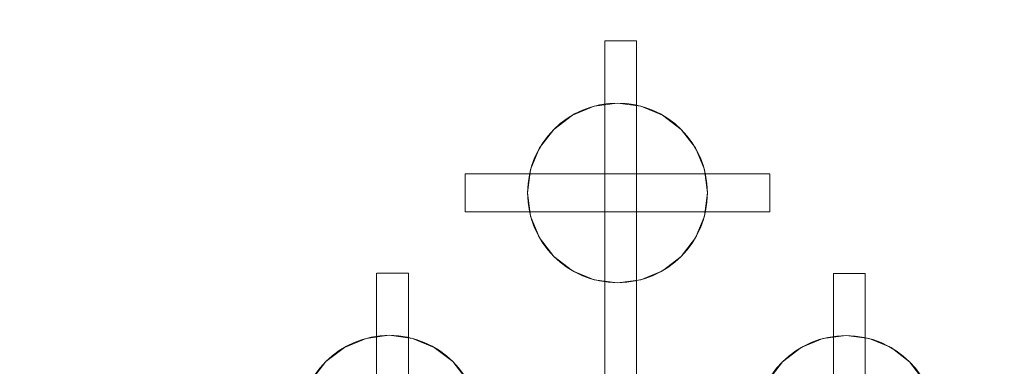
# Model space of a CAD drawing. Units: inches. Extents: x 2696 to 3240, y 1564 to 2310.
# Tile 57 of 76: x 2907.148 to 2916.848, y 2188.894 to 2192.312. Entities that reach past the tile are written whole.
import ezdxf

# ---------------------------------------------------------------- set-up
doc = ezdxf.new("R2010")
doc.units = ezdxf.units.IN
for name, color, linetype, lineweight in [('A-ANNO-DIMS', 3, 'Continuous', 18), ('A-FLOR-FIXT', 8, 'Continuous', 18), ('A-FURN', 251, 'Continuous', 13)]:
    doc.layers.add(name, color=color, linetype=linetype, lineweight=lineweight)
doc.layers.add('FURNITURE', color=250, linetype='Continuous')
doc.styles.add('TIMES NEW', font='times.ttf')
doc.dimstyles.new('Siddhuu', dxfattribs={"dimtxt": 6, "dimasz": 2.5, "dimexe": 1.25, "dimexo": 0.625, "dimtad": 1, "dimdec": 1, "dimlunit": 4, "dimtxsty": 'TIMES NEW', "dimcen": 2.5, "dimclrd": 256, "dimclre": 1, "dimclrt": 7, "dimadec": 0, "dimazin": 0, "dimtfac": 1, "dimtdec": 1, "dimtmove": 0, "dimatfit": 3, "dimfxl": 1, "dimtolj": 1, "dimlwd": -1, "dimarcsym": 0})

# ---------------------------------------------------------------- blocks, each defined once
blk = doc.blocks.new('A$C1af1f523')
at = {"layer": 'A-FURN'}
for p, q in [((-2.9003, 3.9351), (-2.9003, 0.9365)), ((-2.9003, 3.9351, 0.5), (-2.9003, 0.9365, 0.5)), ((-2.9003, 3.9351), (-2.9003, 3.9351, 0.5)), ((-2.5253, 3.9351), (-2.9003, 3.9351)), ((-2.5253, 3.9351, 0.5), (-2.9003, 3.9351, 0.5)), ((-2.5253, 3.9351), (-2.5253, 0.9365)), ((-2.5253, 3.9351, 0.5), (-2.5253, 0.9365, 0.5)), ((-2.5253, 3.9351), (-2.5253, 3.9351, 0.5)), ((-2.7128, 3.3215), (-2.7128, 3.3215, 0.5)), ((-3.1558, 3.2028), (-3.1558, 3.2028, 0.5)), ((-2.9421, 3.2913), (-2.9421, 3.2913, 0.5)), ((-2.4835, 3.2913), (-2.4835, 3.2913, 0.5)), ((-2.2698, 3.2028), (-2.2698, 3.2028, 0.5)), ((-3.3393, 3.062), (-3.3393, 3.062, 0.5)), ((-2.0863, 3.062), (-2.0863, 3.062, 0.5)), ((-3.4801, 2.8785), (-3.4801, 2.8785, 0.5)), ((-1.9455, 2.8785), (-1.9455, 2.8785, 0.5)), ((-3.5686, 2.6648), (-3.5686, 2.6648, 0.5)), ((-1.857, 2.6648), (-1.857, 2.6648, 0.5)), ((0, 2.5605), (-4.2116, 2.5605)), ((0, 2.5605, 0.5), (-4.2116, 2.5605, 0.5)), ((-4.2116, 2.5605), (-4.2116, 2.5605, 0.5)), ((-4.2116, 2.5594), (-4.2116, 2.248)), ((-4.2116, 2.5594, 0.5), (-4.2116, 2.248, 0.5)), ((-4.2116, 2.5594), (-4.2116, 2.5594, 0.5)), ((-3.5988, 2.4355), (-3.5988, 2.4355, 0.5)), ((-1.8268, 2.4355), (-1.8268, 2.4355, 0.5)), ((0, 2.248), (-4.2116, 2.248)), ((0, 2.248, 0.5), (-4.2116, 2.248, 0.5)), ((-4.2116, 2.248), (-4.2116, 2.248, 0.5)), ((-4.2116, 2.248), (-4.2116, 2.2469)), ((-4.2116, 2.248, 0.5), (-4.2116, 2.2469, 0.5)), ((-4.2116, 2.2469), (-4.2116, 2.2469, 0.5)), ((-3.5686, 2.2061), (-3.5686, 2.2061, 0.5)), ((-1.857, 2.2061), (-1.857, 2.2061, 0.5)), ((-3.4801, 1.9924), (-3.4801, 1.9924, 0.5)), ((-1.9455, 1.9924), (-1.9455, 1.9924, 0.5)), ((-3.3393, 1.8089), (-3.3393, 1.8089, 0.5)), ((-2.0863, 1.8089), (-2.0863, 1.8089, 0.5)), ((-4.8156, 1.6871), (-5.1906, 1.6871)), ((-4.8156, 1.6871, 0.5), (-5.1906, 1.6871, 0.5)), ((-5.1906, 1.6871), (-5.1906, 1.6871, 0.5)), ((-5.1906, 1.6871), (-5.1901, -1.3115)), ((-5.1906, 1.6871, 0.5), (-5.1901, -1.3115, 0.5)), ((-4.8156, 1.6871), (-4.8156, 1.6871, 0.5)), ((-4.8156, 1.6871), (-4.8151, -1.3115)), ((-4.8156, 1.6871, 0.5), (-4.8151, -1.3115, 0.5)), ((-3.1558, 1.6681), (-3.1558, 1.6681, 0.5)), ((-2.2698, 1.6681), (-2.2698, 1.6681, 0.5)), ((-2.9421, 1.5796), (-2.9421, 1.5796, 0.5)), ((-2.4835, 1.5796), (-2.4835, 1.5796, 0.5)), ((-2.7128, 1.5494), (-2.7128, 1.5494, 0.5)), ((-5.0026, 1.0735), (-5.0026, 1.0735, 0.5)), ((-5.232, 1.0433), (-5.232, 1.0433, 0.5)), ((-4.7733, 1.0433), (-4.7733, 1.0433, 0.5)), ((-5.4457, 0.9548), (-5.4457, 0.9548, 0.5)), ((-4.5596, 0.9548), (-4.5596, 0.9548, 0.5)), ((-2.9003, 0.9365), (-2.9003, 0.9365, 0.5)), ((-2.5253, 0.9365), (-2.8979, 0.9365)), ((-2.5253, 0.9365, 0.5), (-2.8979, 0.9365, 0.5)), ((-2.8979, 0.9365), (-2.8979, 0.9365, 0.5)), ((-2.5253, 0.9365), (-2.5253, 0.9365, 0.5)), ((-5.6292, 0.814), (-5.6292, 0.814, 0.5)), ((-4.3761, 0.814), (-4.3761, 0.814, 0.5)), ((-5.77, 0.6305), (-5.77, 0.6305, 0.5)), ((-4.2353, 0.6305), (-4.2353, 0.6305, 0.5)), ((-5.8585, 0.4168), (-5.8585, 0.4168, 0.5)), ((-4.1468, 0.4168), (-4.1468, 0.4168, 0.5)), ((0, 0.3125), (-6.5015, 0.3125)), ((0, 0.3125, 0.5), (-6.5015, 0.3125, 0.5)), ((-6.5015, 0.3125), (-6.5015, 0.3125, 0.5)), ((-6.5015, 0.3114), (-6.5015, 0)), ((-6.5015, 0.3114, 0.5), (-6.5015, 0, 0.5)), ((-6.5015, 0.3114), (-6.5015, 0.3114, 0.5)), ((-5.8887, 0.1875), (-5.8887, 0.1875, 0.5)), ((-4.1166, 0.1875), (-4.1166, 0.1875, 0.5)), ((0, 0), (-6.5015, 0)), ((0, 0, 0.5), (-6.5015, 0, 0.5)), ((-6.5015, 0), (-6.5015, 0, 0.5)), ((-6.5015, 0), (-6.5015, -0.0011)), ((-6.5015, 0, 0.5), (-6.5015, -0.0011, 0.5)), ((-6.5015, -0.0011), (-6.5015, -0.0011, 0.5)), ((-5.8585, -0.0418), (-5.8585, -0.0418, 0.5)), ((-4.1468, -0.0418), (-4.1468, -0.0418, 0.5)), ((-5.77, -0.2555), (-5.77, -0.2555, 0.5)), ((-4.2353, -0.2555), (-4.2353, -0.2555, 0.5)), ((-5.6292, -0.439), (-5.6292, -0.439, 0.5)), ((-4.3761, -0.439), (-4.3761, -0.439, 0.5)), ((-5.4457, -0.5798), (-5.4457, -0.5798, 0.5)), ((-4.5596, -0.5798), (-4.5596, -0.5798, 0.5)), ((-2.898, -0.5642), (-2.898, -3.5628)), ((-2.898, -0.5642, 0.5), (-2.898, -3.5628, 0.5)), ((-2.898, -0.5642), (-2.898, -0.5642, 0.5)), ((-2.523, -0.5642), (-2.898, -0.5642)), ((-2.523, -0.5642, 0.5), (-2.898, -0.5642, 0.5)), ((-2.523, -0.5642), (-2.523, -3.5628)), ((-2.523, -0.5642, 0.5), (-2.523, -3.5628, 0.5)), ((-2.523, -0.5642), (-2.523, -0.5642, 0.5)), ((-5.232, -0.6683), (-5.232, -0.6683, 0.5)), ((-4.7733, -0.6683), (-4.7733, -0.6683, 0.5)), ((-5.0026, -0.6985), (-5.0026, -0.6985, 0.5)), ((-2.9398, -1.208), (-2.9398, -1.208, 0.5)), ((-2.7105, -1.1778), (-2.7105, -1.1778, 0.5)), ((-2.4812, -1.208), (-2.4812, -1.208, 0.5)), ((-5.1901, -1.3115), (-5.1901, -1.3115, 0.5)), ((-4.8151, -1.3115), (-5.1878, -1.3115)), ((-4.8151, -1.3115, 0.5), (-5.1878, -1.3115, 0.5)), ((-5.1878, -1.3115), (-5.1878, -1.3115, 0.5)), ((-4.8151, -1.3115), (-4.8151, -1.3115, 0.5)), ((-3.1535, -1.2965), (-3.1535, -1.2965, 0.5)), ((-2.2675, -1.2965), (-2.2675, -1.2965, 0.5)), ((-3.337, -1.4373), (-3.337, -1.4373, 0.5)), ((-2.084, -1.4373), (-2.084, -1.4373, 0.5)), ((-3.4778, -1.6208), (-3.4778, -1.6208, 0.5)), ((-1.9432, -1.6208), (-1.9432, -1.6208, 0.5)), ((-3.5664, -1.8345), (-3.5664, -1.8345, 0.5)), ((-1.8547, -1.8345), (-1.8547, -1.8345, 0.5)), ((0, -1.9388), (-4.2094, -1.9388)), ((0, -1.9388, 0.5), (-4.2094, -1.9388, 0.5)), ((-4.2094, -1.9388), (-4.2094, -1.9388, 0.5)), ((-4.2094, -1.9399), (-4.2094, -2.2513)), ((-4.2094, -1.9399, 0.5), (-4.2094, -2.2513, 0.5)), ((-4.2094, -1.9399), (-4.2094, -1.9399, 0.5)), ((-3.5965, -2.0638), (-3.5965, -2.0638, 0.5)), ((-1.8245, -2.0638), (-1.8245, -2.0638, 0.5)), ((0, -2.2513), (-4.2094, -2.2513)), ((0, -2.2513, 0.5), (-4.2094, -2.2513, 0.5)), ((-4.2094, -2.2513), (-4.2094, -2.2513, 0.5)), ((-4.2094, -2.2513), (-4.2094, -2.2524)), ((-4.2094, -2.2513, 0.5), (-4.2094, -2.2524, 0.5)), ((-4.2094, -2.2524), (-4.2094, -2.2524, 0.5)), ((-3.5664, -2.2931), (-3.5664, -2.2931, 0.5)), ((-1.8547, -2.2931), (-1.8547, -2.2931, 0.5)), ((-3.4778, -2.5068), (-3.4778, -2.5068, 0.5)), ((-1.9432, -2.5068), (-1.9432, -2.5068, 0.5)), ((-3.337, -2.6903), (-3.337, -2.6903, 0.5)), ((-2.084, -2.6903), (-2.084, -2.6903, 0.5)), ((-3.1535, -2.8311), (-3.1535, -2.8311, 0.5)), ((-2.2675, -2.8311), (-2.2675, -2.8311, 0.5)), ((-2.9398, -2.9196), (-2.9398, -2.9196, 0.5)), ((-2.7105, -2.9498), (-2.7105, -2.9498, 0.5)), ((-2.4812, -2.9196), (-2.4812, -2.9196, 0.5)), ((-2.898, -3.5628), (-2.898, -3.5628, 0.5)), ((-2.523, -3.5628), (-2.8956, -3.5628)), ((-2.523, -3.5628, 0.5), (-2.8956, -3.5628, 0.5)), ((-2.8956, -3.5628), (-2.8956, -3.5628, 0.5)), ((-2.523, -3.5628), (-2.523, -3.5628, 0.5))]:
    blk.add_line(p, q, dxfattribs=at)
for centre in [(-2.7128, 2.4355), (-2.7128, 2.4355, 0.5), (-5.0026, 0.1875), (-5.0026, 0.1875, 0.5), (-2.7105, -2.0638), (-2.7105, -2.0638, 0.5)]:
    blk.add_circle(centre, 0.886, dxfattribs=at)
at = {"layer": 'FURNITURE'}
for p, q in [((0, 2.5605), (0, 2.5605, 0.5)), ((0, 2.248), (0, 2.248, 0.5)), ((0, 0.3125), (0, 0.3125, 0.5)), ((0, 0), (0, 0, 0.5)), ((0, -1.9388), (0, -1.9388, 0.5)), ((0, -2.2513), (0, -2.2513, 0.5))]:
    blk.add_line(p, q, dxfattribs=at)
at = {"layer": 'A-FURN'}
mesh = blk.add_polyface(dxfattribs=at)
corners = [(-2.9003, 0.9365, 0.5), (-2.9003, 3.9351), (-2.9003, 0.9365), (-2.9003, 3.9351, 0.5)]
mesh.append_faces([[corners[k] for k in face] for face in [(2, 1, 0), (3, 0, 1)]], dxfattribs={"vtx1": -1})
mesh = blk.add_polyface(dxfattribs=at)
corners = [(-2.5253, 3.9351, 0.5), (-2.9003, 3.9351), (-2.9003, 3.9351, 0.5), (-2.5253, 3.9351)]
mesh.append_faces([[corners[k] for k in face] for face in [(2, 1, 0), (3, 0, 1)]], dxfattribs={"vtx1": -1})
mesh = blk.add_polyface(dxfattribs=at)
corners = [(-2.5253, 0.9365, 0.5), (-2.5253, 3.9351), (-2.5253, 0.9365), (-2.5253, 3.9351, 0.5)]
mesh.append_faces([[corners[k] for k in face] for face in [(2, 1, 0), (3, 0, 1)]], dxfattribs={"vtx1": -1})
mesh = blk.add_polyface(dxfattribs=at)
corners = [(-2.7128, 3.3215), (-2.9421, 3.2913, 0.5), (-2.9421, 3.2913), (-2.7128, 3.3215, 0.5)]
mesh.append_faces([[corners[k] for k in face] for face in [(2, 1, 0), (3, 0, 1)]], dxfattribs={"vtx1": -1})
mesh = blk.add_polyface(dxfattribs=at)
corners = [(-2.4835, 3.2913), (-2.7128, 3.3215, 0.5), (-2.7128, 3.3215), (-2.4835, 3.2913, 0.5)]
mesh.append_faces([[corners[k] for k in face] for face in [(2, 1, 0), (3, 0, 1)]], dxfattribs={"vtx1": -1})
mesh = blk.add_polyface(dxfattribs=at)
corners = [(-3.1558, 3.2028), (-3.3393, 3.062, 0.5), (-3.3393, 3.062), (-3.1558, 3.2028, 0.5)]
mesh.append_faces([[corners[k] for k in face] for face in [(2, 1, 0), (3, 0, 1)]], dxfattribs={"vtx1": -1})
mesh = blk.add_polyface(dxfattribs=at)
corners = [(-2.9421, 3.2913), (-3.1558, 3.2028, 0.5), (-3.1558, 3.2028), (-2.9421, 3.2913, 0.5)]
mesh.append_faces([[corners[k] for k in face] for face in [(2, 1, 0), (3, 0, 1)]], dxfattribs={"vtx1": -1})
mesh = blk.add_polyface(dxfattribs=at)
corners = [(-2.2698, 3.2028), (-2.4835, 3.2913, 0.5), (-2.4835, 3.2913), (-2.2698, 3.2028, 0.5)]
mesh.append_faces([[corners[k] for k in face] for face in [(2, 1, 0), (3, 0, 1)]], dxfattribs={"vtx1": -1})
mesh = blk.add_polyface(dxfattribs=at)
corners = [(-2.0863, 3.062), (-2.2698, 3.2028, 0.5), (-2.2698, 3.2028), (-2.0863, 3.062, 0.5)]
mesh.append_faces([[corners[k] for k in face] for face in [(2, 1, 0), (3, 0, 1)]], dxfattribs={"vtx1": -1})
mesh = blk.add_polyface(dxfattribs=at)
corners = [(-3.3393, 3.062, 0.5), (-3.4801, 2.8785), (-3.3393, 3.062), (-3.4801, 2.8785, 0.5)]
mesh.append_faces([[corners[k] for k in face] for face in [(2, 1, 0), (3, 0, 1)]], dxfattribs={"vtx1": -1})
mesh = blk.add_polyface(dxfattribs=at)
corners = [(-1.9455, 2.8785, 0.5), (-2.0863, 3.062), (-1.9455, 2.8785), (-2.0863, 3.062, 0.5)]
mesh.append_faces([[corners[k] for k in face] for face in [(2, 1, 0), (3, 0, 1)]], dxfattribs={"vtx1": -1})
mesh = blk.add_polyface(dxfattribs=at)
corners = [(-3.4801, 2.8785, 0.5), (-3.5686, 2.6648), (-3.4801, 2.8785), (-3.5686, 2.6648, 0.5)]
mesh.append_faces([[corners[k] for k in face] for face in [(2, 1, 0), (3, 0, 1)]], dxfattribs={"vtx1": -1})
mesh = blk.add_polyface(dxfattribs=at)
corners = [(-1.857, 2.6648, 0.5), (-1.9455, 2.8785), (-1.857, 2.6648), (-1.9455, 2.8785, 0.5)]
mesh.append_faces([[corners[k] for k in face] for face in [(2, 1, 0), (3, 0, 1)]], dxfattribs={"vtx1": -1})
mesh = blk.add_polyface(dxfattribs=at)
corners = [(-3.5686, 2.6648, 0.5), (-3.5988, 2.4355), (-3.5686, 2.6648), (-3.5988, 2.4355, 0.5)]
mesh.append_faces([[corners[k] for k in face] for face in [(2, 1, 0), (3, 0, 1)]], dxfattribs={"vtx1": -1})
mesh = blk.add_polyface(dxfattribs=at)
corners = [(-1.8268, 2.4355, 0.5), (-1.857, 2.6648), (-1.8268, 2.4355), (-1.857, 2.6648, 0.5)]
mesh.append_faces([[corners[k] for k in face] for face in [(2, 1, 0), (3, 0, 1)]], dxfattribs={"vtx1": -1})
mesh = blk.add_polyface(dxfattribs=at)
corners = [(0, 2.5605, 0.5), (-4.2116, 2.5605), (-4.2116, 2.5605, 0.5), (0, 2.5605)]
mesh.append_faces([[corners[k] for k in face] for face in [(2, 1, 0), (3, 0, 1)]], dxfattribs={"vtx1": -1})
mesh = blk.add_polyface(dxfattribs=at)
corners = [(-4.2116, 2.2469, 0.5), (-4.2116, 2.248), (-4.2116, 2.2469), (-4.2116, 2.5594), (-4.2116, 2.5594, 0.5), (-4.2116, 2.248, 0.5)]
mesh.append_faces([[corners[k] for k in face] for face in [(3, 0, 1), (4, 0, 3)]], dxfattribs={"vtx0": -1, "vtx1": -1})
mesh.append_faces([[corners[k] for k in face] for face in [(2, 1, 0), (5, 0, 4)]], dxfattribs={"vtx1": -1})
mesh = blk.add_polyface(dxfattribs=at)
corners = [(-3.5988, 2.4355, 0.5), (-3.5686, 2.2061), (-3.5988, 2.4355), (-3.5686, 2.2061, 0.5)]
mesh.append_faces([[corners[k] for k in face] for face in [(2, 1, 0), (3, 0, 1)]], dxfattribs={"vtx1": -1})
mesh = blk.add_polyface(dxfattribs=at)
corners = [(-1.857, 2.2061, 0.5), (-1.8268, 2.4355), (-1.857, 2.2061), (-1.8268, 2.4355, 0.5)]
mesh.append_faces([[corners[k] for k in face] for face in [(2, 1, 0), (3, 0, 1)]], dxfattribs={"vtx1": -1})
mesh = blk.add_polyface(dxfattribs=at)
corners = [(0, 2.248, 0.5), (-4.2116, 2.248), (-4.2116, 2.248, 0.5), (0, 2.248)]
mesh.append_faces([[corners[k] for k in face] for face in [(2, 1, 0), (3, 0, 1)]], dxfattribs={"vtx1": -1})
mesh = blk.add_polyface(dxfattribs=at)
corners = [(-3.5686, 2.2061, 0.5), (-3.4801, 1.9924), (-3.5686, 2.2061), (-3.4801, 1.9924, 0.5)]
mesh.append_faces([[corners[k] for k in face] for face in [(2, 1, 0), (3, 0, 1)]], dxfattribs={"vtx1": -1})
mesh = blk.add_polyface(dxfattribs=at)
corners = [(-1.9455, 1.9924, 0.5), (-1.857, 2.2061), (-1.9455, 1.9924), (-1.857, 2.2061, 0.5)]
mesh.append_faces([[corners[k] for k in face] for face in [(2, 1, 0), (3, 0, 1)]], dxfattribs={"vtx1": -1})
mesh = blk.add_polyface(dxfattribs=at)
corners = [(-3.4801, 1.9924, 0.5), (-3.3393, 1.8089), (-3.4801, 1.9924), (-3.3393, 1.8089, 0.5)]
mesh.append_faces([[corners[k] for k in face] for face in [(2, 1, 0), (3, 0, 1)]], dxfattribs={"vtx1": -1})
mesh = blk.add_polyface(dxfattribs=at)
corners = [(-2.0863, 1.8089, 0.5), (-1.9455, 1.9924), (-2.0863, 1.8089), (-1.9455, 1.9924, 0.5)]
mesh.append_faces([[corners[k] for k in face] for face in [(2, 1, 0), (3, 0, 1)]], dxfattribs={"vtx1": -1})
mesh = blk.add_polyface(dxfattribs=at)
corners = [(-3.1558, 1.6681, 0.5), (-3.3393, 1.8089), (-3.3393, 1.8089, 0.5), (-3.1558, 1.6681)]
mesh.append_faces([[corners[k] for k in face] for face in [(2, 1, 0), (3, 0, 1)]], dxfattribs={"vtx1": -1})
mesh = blk.add_polyface(dxfattribs=at)
corners = [(-2.0863, 1.8089, 0.5), (-2.2698, 1.6681), (-2.2698, 1.6681, 0.5), (-2.0863, 1.8089)]
mesh.append_faces([[corners[k] for k in face] for face in [(2, 1, 0), (3, 0, 1)]], dxfattribs={"vtx1": -1})
mesh = blk.add_polyface(dxfattribs=at)
corners = [(-4.8156, 1.6871, 0.5), (-5.1906, 1.6871), (-5.1906, 1.6871, 0.5), (-4.8156, 1.6871)]
mesh.append_faces([[corners[k] for k in face] for face in [(2, 1, 0), (3, 0, 1)]], dxfattribs={"vtx1": -1})
mesh = blk.add_polyface(dxfattribs=at)
corners = [(-5.1901, -1.3115, 0.5), (-5.1906, 1.6871), (-5.1901, -1.3115), (-5.1906, 1.6871, 0.5)]
mesh.append_faces([[corners[k] for k in face] for face in [(2, 1, 0), (3, 0, 1)]], dxfattribs={"vtx1": -1})
mesh = blk.add_polyface(dxfattribs=at)
corners = [(-4.8151, -1.3115, 0.5), (-4.8156, 1.6871), (-4.8151, -1.3115), (-4.8156, 1.6871, 0.5)]
mesh.append_faces([[corners[k] for k in face] for face in [(2, 1, 0), (3, 0, 1)]], dxfattribs={"vtx1": -1})
mesh = blk.add_polyface(dxfattribs=at)
corners = [(-2.9421, 1.5796, 0.5), (-3.1558, 1.6681), (-3.1558, 1.6681, 0.5), (-2.9421, 1.5796)]
mesh.append_faces([[corners[k] for k in face] for face in [(2, 1, 0), (3, 0, 1)]], dxfattribs={"vtx1": -1})
mesh = blk.add_polyface(dxfattribs=at)
corners = [(-2.2698, 1.6681, 0.5), (-2.4835, 1.5796), (-2.4835, 1.5796, 0.5), (-2.2698, 1.6681)]
mesh.append_faces([[corners[k] for k in face] for face in [(2, 1, 0), (3, 0, 1)]], dxfattribs={"vtx1": -1})
mesh = blk.add_polyface(dxfattribs=at)
corners = [(-2.7128, 1.5494, 0.5), (-2.9421, 1.5796), (-2.9421, 1.5796, 0.5), (-2.7128, 1.5494)]
mesh.append_faces([[corners[k] for k in face] for face in [(2, 1, 0), (3, 0, 1)]], dxfattribs={"vtx1": -1})
mesh = blk.add_polyface(dxfattribs=at)
corners = [(-2.4835, 1.5796, 0.5), (-2.7128, 1.5494), (-2.7128, 1.5494, 0.5), (-2.4835, 1.5796)]
mesh.append_faces([[corners[k] for k in face] for face in [(2, 1, 0), (3, 0, 1)]], dxfattribs={"vtx1": -1})
mesh = blk.add_polyface(dxfattribs=at)
corners = [(-5.0026, 1.0735), (-5.232, 1.0433, 0.5), (-5.232, 1.0433), (-5.0026, 1.0735, 0.5)]
mesh.append_faces([[corners[k] for k in face] for face in [(2, 1, 0), (3, 0, 1)]], dxfattribs={"vtx1": -1})
mesh = blk.add_polyface(dxfattribs=at)
corners = [(-4.7733, 1.0433), (-5.0026, 1.0735, 0.5), (-5.0026, 1.0735), (-4.7733, 1.0433, 0.5)]
mesh.append_faces([[corners[k] for k in face] for face in [(2, 1, 0), (3, 0, 1)]], dxfattribs={"vtx1": -1})
mesh = blk.add_polyface(dxfattribs=at)
corners = [(-5.232, 1.0433), (-5.4457, 0.9548, 0.5), (-5.4457, 0.9548), (-5.232, 1.0433, 0.5)]
mesh.append_faces([[corners[k] for k in face] for face in [(2, 1, 0), (3, 0, 1)]], dxfattribs={"vtx1": -1})
mesh = blk.add_polyface(dxfattribs=at)
corners = [(-4.5596, 0.9548), (-4.7733, 1.0433, 0.5), (-4.7733, 1.0433), (-4.5596, 0.9548, 0.5)]
mesh.append_faces([[corners[k] for k in face] for face in [(2, 1, 0), (3, 0, 1)]], dxfattribs={"vtx1": -1})
mesh = blk.add_polyface(dxfattribs=at)
corners = [(-5.4457, 0.9548), (-5.6292, 0.814, 0.5), (-5.6292, 0.814), (-5.4457, 0.9548, 0.5)]
mesh.append_faces([[corners[k] for k in face] for face in [(2, 1, 0), (3, 0, 1)]], dxfattribs={"vtx1": -1})
mesh = blk.add_polyface(dxfattribs=at)
corners = [(-4.3761, 0.814), (-4.5596, 0.9548, 0.5), (-4.5596, 0.9548), (-4.3761, 0.814, 0.5)]
mesh.append_faces([[corners[k] for k in face] for face in [(2, 1, 0), (3, 0, 1)]], dxfattribs={"vtx1": -1})
mesh = blk.add_polyface(dxfattribs=at)
corners = [(-2.5253, 0.9365, 0.5), (-2.8979, 0.9365), (-2.8979, 0.9365, 0.5), (-2.5253, 0.9365)]
mesh.append_faces([[corners[k] for k in face] for face in [(2, 1, 0), (3, 0, 1)]], dxfattribs={"vtx1": -1})
mesh = blk.add_polyface(dxfattribs=at)
corners = [(-5.6292, 0.814, 0.5), (-5.77, 0.6305), (-5.6292, 0.814), (-5.77, 0.6305, 0.5)]
mesh.append_faces([[corners[k] for k in face] for face in [(2, 1, 0), (3, 0, 1)]], dxfattribs={"vtx1": -1})
mesh = blk.add_polyface(dxfattribs=at)
corners = [(-4.2353, 0.6305, 0.5), (-4.3761, 0.814), (-4.2353, 0.6305), (-4.3761, 0.814, 0.5)]
mesh.append_faces([[corners[k] for k in face] for face in [(2, 1, 0), (3, 0, 1)]], dxfattribs={"vtx1": -1})
mesh = blk.add_polyface(dxfattribs=at)
corners = [(-5.77, 0.6305, 0.5), (-5.8585, 0.4168), (-5.77, 0.6305), (-5.8585, 0.4168, 0.5)]
mesh.append_faces([[corners[k] for k in face] for face in [(2, 1, 0), (3, 0, 1)]], dxfattribs={"vtx1": -1})
mesh = blk.add_polyface(dxfattribs=at)
corners = [(-4.1468, 0.4168, 0.5), (-4.2353, 0.6305), (-4.1468, 0.4168), (-4.2353, 0.6305, 0.5)]
mesh.append_faces([[corners[k] for k in face] for face in [(2, 1, 0), (3, 0, 1)]], dxfattribs={"vtx1": -1})
mesh = blk.add_polyface(dxfattribs=at)
corners = [(-5.8585, 0.4168, 0.5), (-5.8887, 0.1875), (-5.8585, 0.4168), (-5.8887, 0.1875, 0.5)]
mesh.append_faces([[corners[k] for k in face] for face in [(2, 1, 0), (3, 0, 1)]], dxfattribs={"vtx1": -1})
mesh = blk.add_polyface(dxfattribs=at)
corners = [(-4.1166, 0.1875, 0.5), (-4.1468, 0.4168), (-4.1166, 0.1875), (-4.1468, 0.4168, 0.5)]
mesh.append_faces([[corners[k] for k in face] for face in [(2, 1, 0), (3, 0, 1)]], dxfattribs={"vtx1": -1})
mesh = blk.add_polyface(dxfattribs=at)
corners = [(0, 0.3125, 0.5), (-6.5015, 0.3125), (-6.5015, 0.3125, 0.5), (0, 0.3125)]
mesh.append_faces([[corners[k] for k in face] for face in [(2, 1, 0), (3, 0, 1)]], dxfattribs={"vtx1": -1})
mesh = blk.add_polyface(dxfattribs=at)
corners = [(-6.5015, -0.0011, 0.5), (-6.5015, 0), (-6.5015, -0.0011), (-6.5015, 0.3114), (-6.5015, 0.3114, 0.5), (-6.5015, 0, 0.5)]
mesh.append_faces([[corners[k] for k in face] for face in [(3, 0, 1), (4, 0, 3)]], dxfattribs={"vtx0": -1, "vtx1": -1})
mesh.append_faces([[corners[k] for k in face] for face in [(2, 1, 0), (5, 0, 4)]], dxfattribs={"vtx1": -1})
mesh = blk.add_polyface(dxfattribs=at)
corners = [(-5.8887, 0.1875, 0.5), (-5.8585, -0.0418), (-5.8887, 0.1875), (-5.8585, -0.0418, 0.5)]
mesh.append_faces([[corners[k] for k in face] for face in [(2, 1, 0), (3, 0, 1)]], dxfattribs={"vtx1": -1})
mesh = blk.add_polyface(dxfattribs=at)
corners = [(-4.1468, -0.0418, 0.5), (-4.1166, 0.1875), (-4.1468, -0.0418), (-4.1166, 0.1875, 0.5)]
mesh.append_faces([[corners[k] for k in face] for face in [(2, 1, 0), (3, 0, 1)]], dxfattribs={"vtx1": -1})
mesh = blk.add_polyface(dxfattribs=at)
corners = [(0, 0, 0.5), (-6.5015, 0), (-6.5015, 0, 0.5), (0, 0)]
mesh.append_faces([[corners[k] for k in face] for face in [(2, 1, 0), (3, 0, 1)]], dxfattribs={"vtx1": -1})
mesh = blk.add_polyface(dxfattribs=at)
corners = [(-5.8585, -0.0418, 0.5), (-5.77, -0.2555), (-5.8585, -0.0418), (-5.77, -0.2555, 0.5)]
mesh.append_faces([[corners[k] for k in face] for face in [(2, 1, 0), (3, 0, 1)]], dxfattribs={"vtx1": -1})
mesh = blk.add_polyface(dxfattribs=at)
corners = [(-4.2353, -0.2555, 0.5), (-4.1468, -0.0418), (-4.2353, -0.2555), (-4.1468, -0.0418, 0.5)]
mesh.append_faces([[corners[k] for k in face] for face in [(2, 1, 0), (3, 0, 1)]], dxfattribs={"vtx1": -1})
mesh = blk.add_polyface(dxfattribs=at)
corners = [(-5.77, -0.2555, 0.5), (-5.6292, -0.439), (-5.77, -0.2555), (-5.6292, -0.439, 0.5)]
mesh.append_faces([[corners[k] for k in face] for face in [(2, 1, 0), (3, 0, 1)]], dxfattribs={"vtx1": -1})
mesh = blk.add_polyface(dxfattribs=at)
corners = [(-4.3761, -0.439, 0.5), (-4.2353, -0.2555), (-4.3761, -0.439), (-4.2353, -0.2555, 0.5)]
mesh.append_faces([[corners[k] for k in face] for face in [(2, 1, 0), (3, 0, 1)]], dxfattribs={"vtx1": -1})
mesh = blk.add_polyface(dxfattribs=at)
corners = [(-5.4457, -0.5798, 0.5), (-5.6292, -0.439), (-5.6292, -0.439, 0.5), (-5.4457, -0.5798)]
mesh.append_faces([[corners[k] for k in face] for face in [(2, 1, 0), (3, 0, 1)]], dxfattribs={"vtx1": -1})
mesh = blk.add_polyface(dxfattribs=at)
corners = [(-4.3761, -0.439, 0.5), (-4.5596, -0.5798), (-4.5596, -0.5798, 0.5), (-4.3761, -0.439)]
mesh.append_faces([[corners[k] for k in face] for face in [(2, 1, 0), (3, 0, 1)]], dxfattribs={"vtx1": -1})
mesh = blk.add_polyface(dxfattribs=at)
corners = [(-5.232, -0.6683, 0.5), (-5.4457, -0.5798), (-5.4457, -0.5798, 0.5), (-5.232, -0.6683)]
mesh.append_faces([[corners[k] for k in face] for face in [(2, 1, 0), (3, 0, 1)]], dxfattribs={"vtx1": -1})
mesh = blk.add_polyface(dxfattribs=at)
corners = [(-4.5596, -0.5798, 0.5), (-4.7733, -0.6683), (-4.7733, -0.6683, 0.5), (-4.5596, -0.5798)]
mesh.append_faces([[corners[k] for k in face] for face in [(2, 1, 0), (3, 0, 1)]], dxfattribs={"vtx1": -1})
mesh = blk.add_polyface(dxfattribs=at)
corners = [(-2.898, -3.5628, 0.5), (-2.898, -0.5642), (-2.898, -3.5628), (-2.898, -0.5642, 0.5)]
mesh.append_faces([[corners[k] for k in face] for face in [(2, 1, 0), (3, 0, 1)]], dxfattribs={"vtx1": -1})
mesh = blk.add_polyface(dxfattribs=at)
corners = [(-2.523, -0.5642, 0.5), (-2.898, -0.5642), (-2.898, -0.5642, 0.5), (-2.523, -0.5642)]
mesh.append_faces([[corners[k] for k in face] for face in [(2, 1, 0), (3, 0, 1)]], dxfattribs={"vtx1": -1})
mesh = blk.add_polyface(dxfattribs=at)
corners = [(-2.523, -3.5628, 0.5), (-2.523, -0.5642), (-2.523, -3.5628), (-2.523, -0.5642, 0.5)]
mesh.append_faces([[corners[k] for k in face] for face in [(2, 1, 0), (3, 0, 1)]], dxfattribs={"vtx1": -1})
mesh = blk.add_polyface(dxfattribs=at)
corners = [(-5.0026, -0.6985, 0.5), (-5.232, -0.6683), (-5.232, -0.6683, 0.5), (-5.0026, -0.6985)]
mesh.append_faces([[corners[k] for k in face] for face in [(2, 1, 0), (3, 0, 1)]], dxfattribs={"vtx1": -1})
mesh = blk.add_polyface(dxfattribs=at)
corners = [(-4.7733, -0.6683, 0.5), (-5.0026, -0.6985), (-5.0026, -0.6985, 0.5), (-4.7733, -0.6683)]
mesh.append_faces([[corners[k] for k in face] for face in [(2, 1, 0), (3, 0, 1)]], dxfattribs={"vtx1": -1})
mesh = blk.add_polyface(dxfattribs=at)
corners = [(-2.9398, -1.208), (-3.1535, -1.2965, 0.5), (-3.1535, -1.2965), (-2.9398, -1.208, 0.5)]
mesh.append_faces([[corners[k] for k in face] for face in [(2, 1, 0), (3, 0, 1)]], dxfattribs={"vtx1": -1})
mesh = blk.add_polyface(dxfattribs=at)
corners = [(-2.7105, -1.1778), (-2.9398, -1.208, 0.5), (-2.9398, -1.208), (-2.7105, -1.1778, 0.5)]
mesh.append_faces([[corners[k] for k in face] for face in [(2, 1, 0), (3, 0, 1)]], dxfattribs={"vtx1": -1})
mesh = blk.add_polyface(dxfattribs=at)
corners = [(-2.4812, -1.208), (-2.7105, -1.1778, 0.5), (-2.7105, -1.1778), (-2.4812, -1.208, 0.5)]
mesh.append_faces([[corners[k] for k in face] for face in [(2, 1, 0), (3, 0, 1)]], dxfattribs={"vtx1": -1})
mesh = blk.add_polyface(dxfattribs=at)
corners = [(-2.2675, -1.2965), (-2.4812, -1.208, 0.5), (-2.4812, -1.208), (-2.2675, -1.2965, 0.5)]
mesh.append_faces([[corners[k] for k in face] for face in [(2, 1, 0), (3, 0, 1)]], dxfattribs={"vtx1": -1})
mesh = blk.add_polyface(dxfattribs=at)
corners = [(-4.8151, -1.3115, 0.5), (-5.1878, -1.3115), (-5.1878, -1.3115, 0.5), (-4.8151, -1.3115)]
mesh.append_faces([[corners[k] for k in face] for face in [(2, 1, 0), (3, 0, 1)]], dxfattribs={"vtx1": -1})
mesh = blk.add_polyface(dxfattribs=at)
corners = [(-3.1535, -1.2965), (-3.337, -1.4373, 0.5), (-3.337, -1.4373), (-3.1535, -1.2965, 0.5)]
mesh.append_faces([[corners[k] for k in face] for face in [(2, 1, 0), (3, 0, 1)]], dxfattribs={"vtx1": -1})
mesh = blk.add_polyface(dxfattribs=at)
corners = [(-2.084, -1.4373), (-2.2675, -1.2965, 0.5), (-2.2675, -1.2965), (-2.084, -1.4373, 0.5)]
mesh.append_faces([[corners[k] for k in face] for face in [(2, 1, 0), (3, 0, 1)]], dxfattribs={"vtx1": -1})
mesh = blk.add_polyface(dxfattribs=at)
corners = [(-3.337, -1.4373, 0.5), (-3.4778, -1.6208), (-3.337, -1.4373), (-3.4778, -1.6208, 0.5)]
mesh.append_faces([[corners[k] for k in face] for face in [(2, 1, 0), (3, 0, 1)]], dxfattribs={"vtx1": -1})
mesh = blk.add_polyface(dxfattribs=at)
corners = [(-1.9432, -1.6208, 0.5), (-2.084, -1.4373), (-1.9432, -1.6208), (-2.084, -1.4373, 0.5)]
mesh.append_faces([[corners[k] for k in face] for face in [(2, 1, 0), (3, 0, 1)]], dxfattribs={"vtx1": -1})
mesh = blk.add_polyface(dxfattribs=at)
corners = [(-3.4778, -1.6208, 0.5), (-3.5664, -1.8345), (-3.4778, -1.6208), (-3.5664, -1.8345, 0.5)]
mesh.append_faces([[corners[k] for k in face] for face in [(2, 1, 0), (3, 0, 1)]], dxfattribs={"vtx1": -1})
mesh = blk.add_polyface(dxfattribs=at)
corners = [(-1.8547, -1.8345, 0.5), (-1.9432, -1.6208), (-1.8547, -1.8345), (-1.9432, -1.6208, 0.5)]
mesh.append_faces([[corners[k] for k in face] for face in [(2, 1, 0), (3, 0, 1)]], dxfattribs={"vtx1": -1})
mesh = blk.add_polyface(dxfattribs=at)
corners = [(-3.5664, -1.8345, 0.5), (-3.5965, -2.0638), (-3.5664, -1.8345), (-3.5965, -2.0638, 0.5)]
mesh.append_faces([[corners[k] for k in face] for face in [(2, 1, 0), (3, 0, 1)]], dxfattribs={"vtx1": -1})
mesh = blk.add_polyface(dxfattribs=at)
corners = [(-1.8245, -2.0638, 0.5), (-1.8547, -1.8345), (-1.8245, -2.0638), (-1.8547, -1.8345, 0.5)]
mesh.append_faces([[corners[k] for k in face] for face in [(2, 1, 0), (3, 0, 1)]], dxfattribs={"vtx1": -1})
mesh = blk.add_polyface(dxfattribs=at)
corners = [(0, -1.9388, 0.5), (-4.2094, -1.9388), (-4.2094, -1.9388, 0.5), (0, -1.9388)]
mesh.append_faces([[corners[k] for k in face] for face in [(2, 1, 0), (3, 0, 1)]], dxfattribs={"vtx1": -1})
mesh = blk.add_polyface(dxfattribs=at)
corners = [(-4.2094, -2.2524, 0.5), (-4.2094, -2.2513), (-4.2094, -2.2524), (-4.2094, -1.9399), (-4.2094, -1.9399, 0.5), (-4.2094, -2.2513, 0.5)]
mesh.append_faces([[corners[k] for k in face] for face in [(3, 0, 1), (4, 0, 3)]], dxfattribs={"vtx0": -1, "vtx1": -1})
mesh.append_faces([[corners[k] for k in face] for face in [(2, 1, 0), (5, 0, 4)]], dxfattribs={"vtx1": -1})
mesh = blk.add_polyface(dxfattribs=at)
corners = [(-3.5965, -2.0638, 0.5), (-3.5664, -2.2931), (-3.5965, -2.0638), (-3.5664, -2.2931, 0.5)]
mesh.append_faces([[corners[k] for k in face] for face in [(2, 1, 0), (3, 0, 1)]], dxfattribs={"vtx1": -1})
mesh = blk.add_polyface(dxfattribs=at)
corners = [(-1.8547, -2.2931, 0.5), (-1.8245, -2.0638), (-1.8547, -2.2931), (-1.8245, -2.0638, 0.5)]
mesh.append_faces([[corners[k] for k in face] for face in [(2, 1, 0), (3, 0, 1)]], dxfattribs={"vtx1": -1})
mesh = blk.add_polyface(dxfattribs=at)
corners = [(0, -2.2513, 0.5), (-4.2094, -2.2513), (-4.2094, -2.2513, 0.5), (0, -2.2513)]
mesh.append_faces([[corners[k] for k in face] for face in [(2, 1, 0), (3, 0, 1)]], dxfattribs={"vtx1": -1})
mesh = blk.add_polyface(dxfattribs=at)
corners = [(-3.5664, -2.2931, 0.5), (-3.4778, -2.5068), (-3.5664, -2.2931), (-3.4778, -2.5068, 0.5)]
mesh.append_faces([[corners[k] for k in face] for face in [(2, 1, 0), (3, 0, 1)]], dxfattribs={"vtx1": -1})
mesh = blk.add_polyface(dxfattribs=at)
corners = [(-1.9432, -2.5068, 0.5), (-1.8547, -2.2931), (-1.9432, -2.5068), (-1.8547, -2.2931, 0.5)]
mesh.append_faces([[corners[k] for k in face] for face in [(2, 1, 0), (3, 0, 1)]], dxfattribs={"vtx1": -1})
mesh = blk.add_polyface(dxfattribs=at)
corners = [(-3.4778, -2.5068, 0.5), (-3.337, -2.6903), (-3.4778, -2.5068), (-3.337, -2.6903, 0.5)]
mesh.append_faces([[corners[k] for k in face] for face in [(2, 1, 0), (3, 0, 1)]], dxfattribs={"vtx1": -1})
mesh = blk.add_polyface(dxfattribs=at)
corners = [(-2.084, -2.6903, 0.5), (-1.9432, -2.5068), (-2.084, -2.6903), (-1.9432, -2.5068, 0.5)]
mesh.append_faces([[corners[k] for k in face] for face in [(2, 1, 0), (3, 0, 1)]], dxfattribs={"vtx1": -1})
mesh = blk.add_polyface(dxfattribs=at)
corners = [(-3.1535, -2.8311, 0.5), (-3.337, -2.6903), (-3.337, -2.6903, 0.5), (-3.1535, -2.8311)]
mesh.append_faces([[corners[k] for k in face] for face in [(2, 1, 0), (3, 0, 1)]], dxfattribs={"vtx1": -1})
mesh = blk.add_polyface(dxfattribs=at)
corners = [(-2.084, -2.6903, 0.5), (-2.2675, -2.8311), (-2.2675, -2.8311, 0.5), (-2.084, -2.6903)]
mesh.append_faces([[corners[k] for k in face] for face in [(2, 1, 0), (3, 0, 1)]], dxfattribs={"vtx1": -1})
mesh = blk.add_polyface(dxfattribs=at)
corners = [(-2.9398, -2.9196, 0.5), (-3.1535, -2.8311), (-3.1535, -2.8311, 0.5), (-2.9398, -2.9196)]
mesh.append_faces([[corners[k] for k in face] for face in [(2, 1, 0), (3, 0, 1)]], dxfattribs={"vtx1": -1})
mesh = blk.add_polyface(dxfattribs=at)
corners = [(-2.2675, -2.8311, 0.5), (-2.4812, -2.9196), (-2.4812, -2.9196, 0.5), (-2.2675, -2.8311)]
mesh.append_faces([[corners[k] for k in face] for face in [(2, 1, 0), (3, 0, 1)]], dxfattribs={"vtx1": -1})
mesh = blk.add_polyface(dxfattribs=at)
corners = [(-2.7105, -2.9498, 0.5), (-2.9398, -2.9196), (-2.9398, -2.9196, 0.5), (-2.7105, -2.9498)]
mesh.append_faces([[corners[k] for k in face] for face in [(2, 1, 0), (3, 0, 1)]], dxfattribs={"vtx1": -1})
mesh = blk.add_polyface(dxfattribs=at)
corners = [(-2.4812, -2.9196, 0.5), (-2.7105, -2.9498), (-2.7105, -2.9498, 0.5), (-2.4812, -2.9196)]
mesh.append_faces([[corners[k] for k in face] for face in [(2, 1, 0), (3, 0, 1)]], dxfattribs={"vtx1": -1})
mesh = blk.add_polyface(dxfattribs=at)
corners = [(-2.523, -3.5628, 0.5), (-2.8956, -3.5628), (-2.8956, -3.5628, 0.5), (-2.523, -3.5628)]
mesh.append_faces([[corners[k] for k in face] for face in [(2, 1, 0), (3, 0, 1)]], dxfattribs={"vtx1": -1})
blk = doc.blocks.new('*D59')
at = {"layer": 'A-ANNO-DIMS', "color": 1, "lineweight": -2, "transparency": 16777216}
for p, q in [((2884.7088, 1740.8261), (2884.7088, 2298.4511)), ((2956.7088, 1740.8261), (2956.7088, 2298.4511))]:
    blk.add_line(p, q, dxfattribs=at)
at = {"layer": 'A-ANNO-DIMS', "transparency": 16777216}
blk.add_line((2887.2088, 2297.2011), (2954.2088, 2297.2011), dxfattribs=at)
for points in [[(2887.2088, 2297.6178), (2887.2088, 2296.7844), (2884.7088, 2297.2011)], [(2954.2088, 2297.6178), (2954.2088, 2296.7844), (2956.7088, 2297.2011)]]:
    blk.add_solid(points, dxfattribs=at)
at = {"layer": 'Defpoints', "color": 0, "transparency": 16777216}
for p in [(2956.7088, 2297.2011), (2884.7088, 1740.2011), (2956.7088, 1740.2011)]:
    blk.add_point(p, dxfattribs=at)
at = {"layer": 'A-ANNO-DIMS', "color": 7, "transparency": 16777216, "insert": (2920.7088, 2300.878), "char_height": 6, "attachment_point": 5, "style": 'TIMES NEW'}
blk.add_mtext('\\A1;6\'-0"', dxfattribs=at)
blk = doc.blocks.new('*D64')
at = {"layer": 'A-ANNO-DIMS', "color": 1, "lineweight": -2, "transparency": 16777216}
for p, q in [((3073.0838, 2206.7011), (2709.3614, 2206.7011)), ((3068.5838, 1989.2011), (2709.3614, 1989.2011))]:
    blk.add_line(p, q, dxfattribs=at)
at = {"layer": 'A-ANNO-DIMS', "transparency": 16777216}
blk.add_line((2710.6114, 1991.7011), (2710.6114, 2204.2011), dxfattribs=at)
for points in [[(2710.1947, 2204.2011), (2711.0281, 2204.2011), (2710.6114, 2206.7011)], [(2710.1947, 1991.7011), (2711.0281, 1991.7011), (2710.6114, 1989.2011)]]:
    blk.add_solid(points, dxfattribs=at)
at = {"layer": 'Defpoints', "color": 0, "transparency": 16777216}
for p in [(2710.6114, 2206.7011), (3073.7088, 2206.7011), (3069.2088, 1989.2011)]:
    blk.add_point(p, dxfattribs=at)
at = {"layer": 'A-ANNO-DIMS', "color": 7, "transparency": 16777216, "insert": (2706.8501, 2097.9511), "char_height": 6, "attachment_point": 5, "rotation": 90, "style": 'TIMES NEW'}
blk.add_mtext('\\A1;18\'-1 1/2"', dxfattribs=at)

msp = doc.modelspace()

# ---------------------------------------------------------------- block references
at = {"layer": 'A-FLOR-FIXT', "xscale": -1, "rotation": 90}
msp.add_blockref('A$C1af1f523', (2913.2252, 2185.6011), dxfattribs=at)

# ---------------------------------------------------------------- dimensions: what is measured, and where the dimension line sits
at = {"layer": 'A-ANNO-DIMS'}
dim = msp.add_linear_dim(base=(2956.7088, 2297.2011), p1=(2884.7088, 1740.2011), p2=(2956.7088, 1740.2011), dimstyle='Siddhuu', override={"dimdec": 1, "dimlfac": 1, "dimrnd": 0, "dimzin": 1, "dimdsep": 46, "dimlunit": 4, "dimfrac": 2}, dxfattribs=at)
dim.commit()
dim.dimension.update_dxf_attribs({"geometry": '*D59', "text_midpoint": (2920.7088, 2300.878)})
dim = msp.add_linear_dim(base=(2710.6114, 2206.7011), p1=(3069.2088, 1989.2011), p2=(3073.7088, 2206.7011), angle=90, dimstyle='Siddhuu', override={"dimdec": 1, "dimlfac": 1, "dimrnd": 0, "dimzin": 1, "dimdsep": 46, "dimlunit": 4, "dimfrac": 2}, dxfattribs=at)
dim.commit()
dim.dimension.update_dxf_attribs({"geometry": '*D64', "text_midpoint": (2706.8501, 2097.9511)})

doc.saveas('drawing.dxf')
